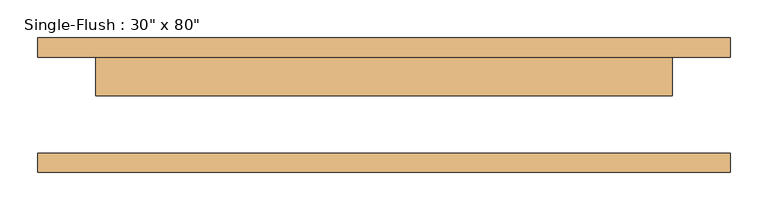
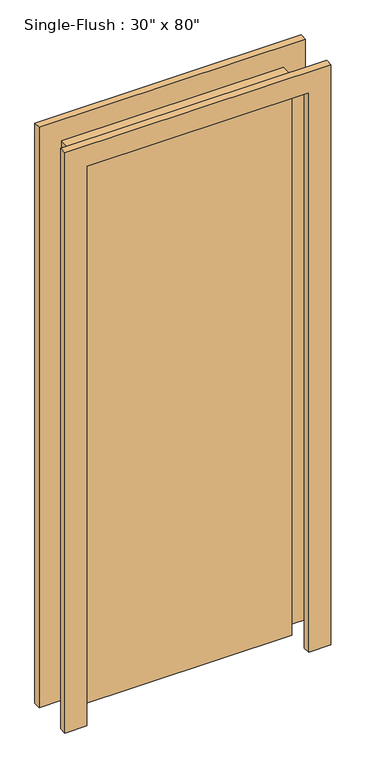
"""IFC4 building model written with IfcOpenShell, lengths in millimetres: door geometry."""

from ifc_helpers import new_model, si_unit, frame, origin, origin_with_axes, place, context, project, spatial, polyline, outline, extrude, source, transform, mapped, element, save


def door_1fe7f57d(model_context):
    return source(origin(), model_context, "Body", "SweptSolid", [
        extrude(outline(polyline([(2108.2, -457.2), (0.0, -457.2), (0.0, -381.0), (2032.0, -381.0), (2032.0, 381.0), (0.0, 381.0), (0.0, 457.2), (2108.2, 457.2), (2108.2, -457.2)])), frame((0.0, 63.5, 0.0), z_axis=(0.0, 1.0, 0.0), x_axis=(0.0, 0.0, 1.0)), (0.0, 0.0, 1.0), 25.4),
        extrude(outline(polyline([(2108.2, 457.2), (2108.2, -457.2), (0.0, -457.2), (0.0, -381.0), (2032.0, -381.0), (2032.0, 381.0), (0.0, 381.0), (0.0, 457.2), (2108.2, 457.2)])), frame((0.0, -88.9, 0.0), z_axis=(0.0, 1.0, 0.0), x_axis=(0.0, 0.0, 1.0)), (0.0, 0.0, 1.0), 25.4),
        extrude(outline(polyline([(381.0, 12.7), (-381.0, 12.7), (-381.0, 63.5), (381.0, 63.5), (381.0, 12.7)])), origin_with_axes(), (0.0, 0.0, 1.0), 2032.0),
    ])


if __name__ == "__main__":
    model = new_model("IFC4")
    model_context = context("Model", 3, world=origin())
    ifc_project = project(units=[si_unit("LENGTHUNIT", "METRE", prefix="MILLI")], contexts=[model_context])
    site = spatial("IfcSite", under=ifc_project)
    building = spatial("IfcBuilding", under=site)
    placement = place(None, origin())
    door_shape = door_1fe7f57d(model_context)
    element("IfcDoor", 1, ObjectType="Single-Flush : 30\" x 80\"", at=placement, inside=building, context=model_context, shape_type="MappedRepresentation", body=[
        mapped(door_shape, transform((0.0, 0.0, 0.0), x_axis=(1.0, 0.0, 0.0), y_axis=(0.0, 1.0, 0.0), z_axis=(0.0, 0.0, 1.0))),
    ])
    save(model, "model.ifc")

# Revit data of these elements
# Type "Single-Flush : 30\" x 80\""
#   Type Mark = "5"
#   Construction Type Id = "MDOOR"
#   Assembly Code = "C1020"
#   Analytic Construction = "Metal"
#   Thickness = 0' - 2"
#   Heat Transfer Coefficient (U) = 0.651978 BTU/(h·ft²·°F)
#   Height = 6' - 8"
#   Trim Projection Ext = 0' - 1"
#   Trim Projection Int = 0' - 1"
#   Trim Width = 0' - 3"
#   Width = 2' - 6"
#   Define Thermal Properties by = 1
#   Define Thermal Properties by = 1
#   Door Material = Door - Panel
#   Frame Material = Door - Frame
#   Visual Light Transmittance = 0
#   Solar Heat Gain Coefficient = 0
#   Function = (empty or 0)
#   Wall Closure = (empty or 0)
# Element 1 (IfcDoor, "Single-Flush : 30\" x 80\"")
#   Materials on its faces: "Door - Frame", "Door - Panel"
# Materials
#   "Door - Panel": class "Wood", colour RGB 210 159 95, transparency 0, Cost = 0
#   "Door - Frame": colour RGB 118 70 51, transparency 0, Cost = 0
